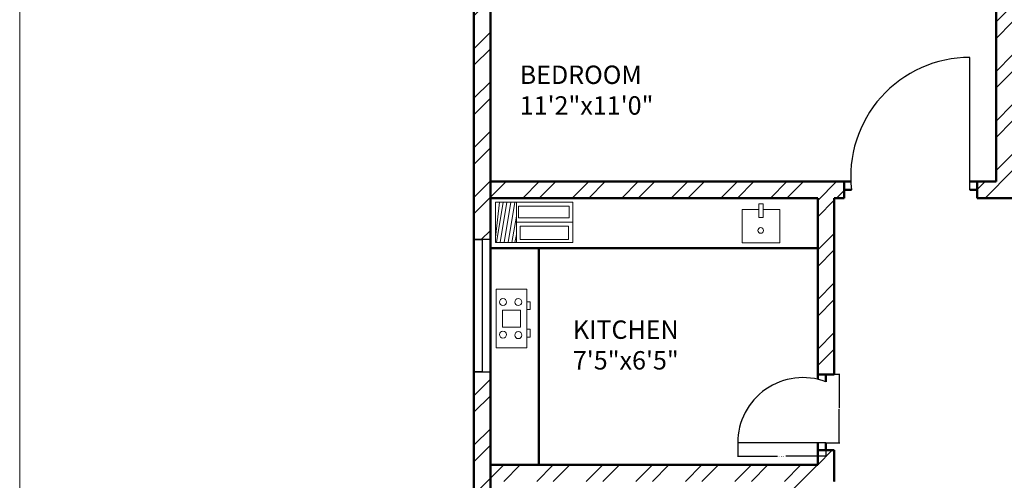
# Model space of a CAD drawing. Units: inches. Extents: x 1901 to 2863, y 888 to 2433.
# Tile 54 of 91: x 1901 to 2169, y 2002 to 2127. Entities that reach past the tile are written whole.
import ezdxf

# ---------------------------------------------------------------- set-up
doc = ezdxf.new("R2010")
doc.units = ezdxf.units.IN
for name, color, linetype, lineweight in [('A-ANNO-DIMS', 2, 'Continuous', 18), ('A-AREA-IDEN', 7, 'Continuous', 18), ('A-DOOR', 4, 'Continuous', 25), ('A-FLOR-FIXT', 9, 'Continuous', 18), ('A-GLAZ', 3, 'Continuous', 25), ('A-WALL', 7, 'Continuous', 50), ('A-WALL-PATT', 8, 'Continuous', 13)]:
    doc.layers.add(name, color=color, linetype=linetype, lineweight=lineweight)
doc.styles.get("Standard").update_dxf_attribs({"font": 'arial.ttf'})
doc.dimstyles.get("Standard").update_dxf_attribs({"dimtxt": 0.18, "dimasz": 0.18, "dimexe": 0.18, "dimexo": 0.0625, "dimgap": 0.09, "dimtad": 0, "dimtih": 1, "dimtoh": 1, "dimdec": 4, "dimzin": 0, "dimdsep": 46, "dimtxsty": 'Standard', "dimcen": 0.09, "dimadec": 0, "dimazin": 0, "dimtfac": 1, "dimtdec": 4, "dimtofl": 0, "dimtmove": 0, "dimatfit": 3, "dimfxl": 1, "dimtolj": 1, "dimtzin": 0, "dimarcsym": 0})

# ---------------------------------------------------------------- blocks, each defined once
blk = doc.blocks.new('WIN-36')
for p, q in [((4.5, 36), (0, 36)), ((0, 36), (2.25, 36)), ((2.25, 36), (2.25, 0)), ((2.25, 0), (0, 0)), ((0, 0), (4.5, 0))]:
    blk.add_line(p, q)
blk = doc.blocks.new('DOOR-18')
blk.add_line((23.98, -0.01), (-0.02, -0.01))
blk.add_arc((17.74, -0.01), 17.76, 69.4255, 180)
blk = doc.blocks.new('*D41')
at = {"layer": 'A-ANNO-DIMS', "color": 0, "lineweight": -2, "transparency": 16777216}
for p, q in [((2096.68, 2012.03), (2096.68, 2008.31)), ((2120.68, 2012.03), (2120.68, 2008.31)), ((2096.86, 2008.49), (2107.54, 2008.49)), ((2120.5, 2008.49), (2109.81, 2008.49))]:
    blk.add_line(p, q, dxfattribs=at)
at = {"layer": 'A-ANNO-DIMS', "color": 0, "transparency": 16777216}
for points in [[(2096.86, 2008.52), (2096.86, 2008.46), (2096.68, 2008.49)], [(2120.5, 2008.52), (2120.5, 2008.46), (2120.68, 2008.49)]]:
    blk.add_solid(points, dxfattribs=at)
at = {"layer": 'Defpoints', "color": 0, "transparency": 16777216}
for p in [(2096.68, 2012.09), (2120.68, 2012.09), (2120.68, 2008.49)]:
    blk.add_point(p, dxfattribs=at)
at = {"layer": 'A-ANNO-DIMS', "color": 0, "transparency": 16777216, "insert": (2108.68, 2008.49), "char_height": 0.18, "attachment_point": 5}
blk.add_mtext('\\A1;DOOR D6 24 TYP.', dxfattribs=at)
blk = doc.blocks.new('*D42')
at = {"layer": 'A-ANNO-DIMS', "color": 0, "lineweight": -2, "transparency": 16777216}
for p, q in [((2120.74, 2030.76), (2124.46, 2030.76)), ((2124.28, 2030.58), (2124.28, 2021.61)), ((2124.28, 2012.27), (2124.28, 2021.24)), ((2120.74, 2012.09), (2124.46, 2012.09))]:
    blk.add_line(p, q, dxfattribs=at)
at = {"layer": 'A-ANNO-DIMS', "color": 0, "transparency": 16777216}
for points in [[(2124.25, 2030.58), (2124.31, 2030.58), (2124.28, 2030.76)], [(2124.25, 2012.27), (2124.31, 2012.27), (2124.28, 2012.09)]]:
    blk.add_solid(points, dxfattribs=at)
at = {"layer": 'Defpoints', "color": 0, "transparency": 16777216}
for p in [(2120.68, 2030.76), (2124.28, 2030.76), (2120.68, 2012.09)]:
    blk.add_point(p, dxfattribs=at)
at = {"layer": 'A-ANNO-DIMS', "color": 0, "transparency": 16777216, "insert": (2124.28, 2021.43), "char_height": 0.18, "attachment_point": 5}
blk.add_mtext('\\A1;19 TYP.', dxfattribs=at)

msp = doc.modelspace()

# ---------------------------------------------------------------- hatches: boundary and pattern name
at = {"layer": 'A-WALL-PATT'}
h = msp.add_hatch(dxfattribs=at)
h.set_pattern_fill('ANSI32', color=256)
h.paths.add_polyline_path([(2192.5, 2274.13), (2141.26, 2274.13), (2141.26, 2269.63), (2192.5, 2269.63)])
h.paths.add_polyline_path([(2259.93, 2274.13), (2216.5, 2274.13), (2216.5, 2269.63), (2255.43, 2269.63), (2255.43, 2214.63), (2250.81, 2214.63), (2250.81, 2210.13), (2259.93, 2210.13), (2259.93, 2215.13), (2271.76, 2215.13), (2271.76, 2217.38), (2271.76, 2219.63), (2259.93, 2219.63)])
h.paths.add_polyline_path([(2171.43, 2269.63), (2166.93, 2269.63), (2166.93, 2219.63), (2121.24, 2219.63), (2121.24, 2215.13), (2166.93, 2215.13), (2166.93, 2083.13), (2161.81, 2083.13), (2161.81, 2078.63), (2171.43, 2078.63), (2177, 2078.63), (2177, 2080.88), (2177, 2083.13), (2171.43, 2083.13), (2171.43, 2210.13), (2230.91, 2210.13), (2230.91, 2212.38), (2230.91, 2214.63), (2171.43, 2214.63)])
h.paths.add_polyline_path([(2117.26, 2274.13), (2089.43, 2274.13), (2089.43, 2219.63), (2081.14, 2219.63), (2081.14, 2215.13), (2089.43, 2215.13), (2098, 2215.13), (2098, 2217.38), (2098, 2219.63), (2093.93, 2219.63), (2093.93, 2269.63), (2117.26, 2269.63), (2117.26, 2271.88)])
h.paths.add_polyline_path([(2343.43, 2219.63), (2329.29, 2219.63), (2329.29, 2215.13), (2338.93, 2215.13), (2338.93, 2184.74), (2343.43, 2184.74)])
h.paths.add_polyline_path([(2338.93, 2083.13), (2329.29, 2083.13), (2208.97, 2083.13), (2208.97, 2078.63), (2338.93, 2078.63)])
h.paths.add_polyline_path([(2343.43, 2136.74), (2338.93, 2136.74), (2338.93, 1872.63), (2343.43, 1872.63)])
h.paths.add_polyline_path([(2343.43, 1863.63), (2397.68, 1863.63), (2397.68, 1821.63), (2384.14, 1821.63), (2384.14, 1812.63), (2418.33, 1812.63), (2418.33, 1817.13), (2418.33, 1821.63), (2406.68, 1821.63), (2406.68, 1863.63), (2459.5, 1863.63), (2459.5, 1821.63), (2447.14, 1821.63), (2447.14, 1812.63), (2459.5, 1812.63), (2468.5, 1812.63), (2468.5, 1872.63), (2394.43, 1872.63), (2334.43, 1872.63), (2334.43, 1812.63), (2343.43, 1812.63), (2353.25, 1812.63), (2353.25, 1821.63), (2343.43, 1821.63)])
h.paths.add_polyline_path([(2510.01, 1872.63), (2468.5, 1872.63), (2468.5, 1868.13), (2510.01, 1868.13)])
h.paths.add_polyline_path([(2514.01, 1817.13), (2468.5, 1817.13), (2468.5, 1812.63), (2482.11, 1812.63), (2482.11, 1800.61), (2486.61, 1800.61), (2486.61, 1812.63), (2514.01, 1812.63)])
h.paths.add_polyline_path([(2299.25, 1814.88), (2299.25, 1817.13), (2295.93, 1817.13), (2295.93, 1854.17), (2293.68, 1854.17), (2291.43, 1854.17), (2291.43, 1817.13), (2266.11, 1817.13), (2266.11, 1812.63), (2299.25, 1812.63)])
h.paths.add_polyline_path([(2218.11, 1817.13), (2206.46, 1817.13), (2171.43, 1817.13), (2171.43, 1949.13), (2190.1, 1949.13), (2190.1, 1953.63), (2163.47, 1953.63), (2163.47, 1949.13), (2166.93, 1949.13), (2166.93, 1817.13), (2114.3, 1817.13), (2114.3, 1812.63), (2218.11, 1812.63)])
h.paths.add_polyline_path([(2029.43, 1970.92), (2024.93, 1970.92), (2024.93, 1912.72), (2029.43, 1912.72)])
h.paths.add_polyline_path([(2132.3, 1953.63), (2113.93, 1953.63), (2113.93, 1975.89), (2111.68, 1975.89), (2109.43, 1975.89), (2109.43, 1953.63), (2029.43, 1953.63), (2029.43, 1949.13), (2132.3, 1949.13)])
h.paths.add_polyline_path([(2029.43, 1853.61), (2029.31, 1853.61), (2029.31, 1853.61), (2029.43, 1853.61), (2029.43, 1864.72), (2024.93, 1864.72), (2024.93, 1812.63), (2066.3, 1812.63), (2066.3, 1814.88), (2066.3, 1817.13), (2029.43, 1817.13)])
h.paths.add_polyline_path([(2122.93, 2010.09), (2120.68, 2010.09), (2118.43, 2010.09), (2118.43, 2006.13), (2029.43, 2006.13), (2029.43, 2001.63), (2109.43, 2001.63), (2109.43, 1998.04), (2113.93, 1998.04), (2113.93, 2001.63), (2122.93, 2001.63)])
h.paths.add_polyline_path([(2029.43, 2031.38), (2024.93, 2031.38), (2024.93, 1994.92), (2027.18, 1994.92), (2029.43, 1994.92)])
h.paths.add_polyline_path([(2029.43, 2136.74), (2024.93, 2136.74), (2024.93, 2067.38), (2027.18, 2067.38), (2029.43, 2067.38)])
h.paths.add_polyline_path([(2125.62, 2083.13), (2029.43, 2083.13), (2029.43, 2078.63), (2118.43, 2078.63), (2118.43, 2030.71), (2122.93, 2030.71), (2122.93, 2078.63), (2125.62, 2078.63)])
h.paths.add_polyline_path([(2029.43, 2215.13), (2040.47, 2215.13), (2040.47, 2217.38), (2040.47, 2219.63), (2024.93, 2219.63), (2024.93, 2184.74), (2029.43, 2184.74), (2029.43, 2187.78)])
h.paths.add_polyline_path([(2686.43, 2274.13), (2659.28, 2274.13), (2659.28, 2269.63), (2681.93, 2269.63), (2681.93, 2219.63), (2676.82, 2219.63), (2676.82, 2215.13), (2681.93, 2215.13), (2697.01, 2215.13), (2697.01, 2217.38), (2697.01, 2219.63), (2686.43, 2219.63)])
h.paths.add_polyline_path([(2609.93, 2269.63), (2635.28, 2269.63), (2635.28, 2274.13), (2571.43, 2274.13), (2571.43, 2269.63), (2605.43, 2269.63), (2605.43, 2214.63), (2549.1, 2214.63), (2549.1, 2210.13), (2605.43, 2210.13), (2605.43, 2083.13), (2601.01, 2083.13), (2601.01, 2080.88), (2601.01, 2078.63), (2609.93, 2078.63), (2616.16, 2078.63), (2616.16, 2080.88), (2616.16, 2083.13), (2609.93, 2083.13), (2609.93, 2215.13), (2651.46, 2215.13), (2651.46, 2217.38), (2651.46, 2219.63), (2609.93, 2219.63)])
h.paths.add_polyline_path([(2521.43, 2269.63), (2547.43, 2269.63), (2547.43, 2271.88), (2547.43, 2274.13), (2516.93, 2274.13), (2516.93, 2219.63), (2506.41, 2219.63), (2506.41, 2215.13), (2516.93, 2215.13), (2516.93, 2210.13), (2525.4, 2210.13), (2525.4, 2212.38), (2525.4, 2214.63), (2521.43, 2214.63)])
h.paths.add_polyline_path([(2456.01, 2219.63), (2439.43, 2219.63), (2439.43, 2187.89), (2443.93, 2187.89), (2443.93, 2215.13), (2456.01, 2215.13)])
h.paths.add_polyline_path([(2752.93, 2219.63), (2739.48, 2219.63), (2739.48, 2215.13), (2748.43, 2215.13), (2748.43, 2187.89), (2752.93, 2187.89)])
h.paths.add_polyline_path([(2752.93, 2139.89), (2748.43, 2139.89), (2748.43, 2083.13), (2648.42, 2083.13), (2648.42, 2078.63), (2654.93, 2078.63), (2654.93, 2039.44), (2659.43, 2039.44), (2659.43, 2078.63), (2748.43, 2078.63), (2748.43, 2063.43), (2752.93, 2063.43)])
h.paths.add_polyline_path([(2752.93, 2010.63), (2659.43, 2010.63), (2659.43, 2015.65), (2654.93, 2015.65), (2654.93, 2010.63), (2605.43, 2010.63), (2605.43, 1920.97), (2609.93, 1920.97), (2609.93, 2006.13), (2748.43, 2006.13), (2748.43, 1982.47), (2752.93, 1982.47)])
h.paths.add_polyline_path([(2752.93, 2027.43), (2748.43, 2027.43), (2748.43, 2010.63), (2752.93, 2010.63)])
h.paths.add_polyline_path([(2748.43, 1886.13), (2609.93, 1886.13), (2609.93, 1889.72), (2605.43, 1889.72), (2605.43, 1861.26), (2609.93, 1861.26), (2609.93, 1881.63), (2748.43, 1881.63)])
h.paths.add_polyline_path([(2456.86, 2228.83), (2498.4, 2228.83), (2498.4, 2247.49), (2456.86, 2247.49)], flags=9)
h.paths.add_polyline_path([(2038.6, 2237.42), (2080.17, 2237.42), (2080.17, 2256.08), (2038.6, 2256.08)], flags=9)
h.paths.add_polyline_path([(2292.01, 1062.39), (2539.93, 1062.39), (2539.93, 1099.49), (2292.01, 1099.49)], flags=9)
h.paths.add_polyline_path([(2424.91, 1832.25), (2448.51, 1832.25), (2448.51, 1846.68), (2424.91, 1846.68)], flags=25)
h.paths.add_polyline_path([(2359.08, 1832.25), (2382.68, 1832.25), (2382.68, 1846.68), (2359.08, 1846.68)], flags=25)
h.paths.add_polyline_path([(2352.9, 1684.8), (2367.54, 1684.8), (2367.54, 1697.17), (2352.9, 1697.17)], flags=9)
h.paths.add_polyline_path([(2079.29, 1755.83), (2169.02, 1755.83), (2169.02, 1774.37), (2079.29, 1774.37)], flags=9)
h.paths.add_polyline_path([(2404.09, 1373.86), (2404.09, 1463.59), (2385.54, 1463.59), (2385.54, 1373.86)], flags=9)
h.paths.add_polyline_path([(2268.09, 2236.37), (2309.64, 2236.37), (2309.64, 2255.03), (2268.09, 2255.03)], flags=9)
h.paths.add_polyline_path([(2575.96, 1700.95), (2665.7, 1700.95), (2665.7, 1719.5), (2575.96, 1719.5)], flags=9)
h.paths.add_polyline_path([(2302.96, 1878.47), (2329.52, 1878.47), (2329.52, 1888.78), (2302.96, 1888.78)], flags=9)
h.paths.add_polyline_path([(2097.42, 2240.58), (2126.57, 2240.58), (2126.57, 2259.23), (2097.42, 2259.23)], flags=9)
h.paths.add_polyline_path([(2208.72, 2246.12), (2237.88, 2246.12), (2237.88, 2264.78), (2208.72, 2264.78)], flags=9)
h.paths.add_polyline_path([(2038.15, 1925.96), (2076.99, 1925.96), (2076.99, 1944.62), (2038.15, 1944.62)], flags=9)
h.paths.add_polyline_path([(2239.14, 1926.67), (2288.46, 1926.67), (2288.46, 1945.33), (2239.14, 1945.33)], flags=9)
h.paths.add_polyline_path([(2175.43, 2007.33), (2212.36, 2007.33), (2212.36, 2025.99), (2175.43, 2025.99)], flags=9)
h.paths.add_polyline_path([(2225.03, 2091.79), (2263.87, 2091.79), (2263.87, 2110.45), (2225.03, 2110.45)], flags=9)
h.paths.add_polyline_path([(2035.4, 2098.48), (2074.24, 2098.48), (2074.24, 2117.14), (2035.4, 2117.14)], flags=9)
h.paths.add_polyline_path([(2050.1, 2029.21), (2083.26, 2029.21), (2083.26, 2047.87), (2050.1, 2047.87)], flags=9)
h.paths.add_polyline_path([(2069.68, 1956.72), (2098.83, 1956.72), (2098.83, 1975.38), (2069.68, 1975.38)], flags=25)
h.paths.add_polyline_path([(2328.62, 1753.34), (2361.66, 1753.34), (2361.66, 1771.99), (2328.62, 1771.99)], flags=9)
h.paths.add_polyline_path([(2395.16, 2060.89), (2395.16, 2140.65), (2378.68, 2140.65), (2378.68, 2060.89)], flags=9)
h.paths.add_polyline_path([(2463.73, 2059.02), (2492.89, 2059.02), (2492.89, 2077.68), (2463.73, 2077.68)], flags=9)
h.paths.add_polyline_path([(2458.03, 2181.54), (2496.87, 2181.54), (2496.87, 2200.19), (2458.03, 2200.19)], flags=9)
h.paths.add_polyline_path([(2527.58, 2243.07), (2556.73, 2243.07), (2556.73, 2261.73), (2527.58, 2261.73)], flags=9)
h.paths.add_polyline_path([(2694.46, 2232.77), (2736.03, 2232.77), (2736.03, 2251.42), (2694.46, 2251.42)], flags=9)
h.paths.add_polyline_path([(2637.82, 2249.22), (2666.98, 2249.22), (2666.98, 2267.88), (2637.82, 2267.88)], flags=9)
h.paths.add_polyline_path([(2623.69, 2183.54), (2662.53, 2183.54), (2662.53, 2202.2), (2623.69, 2202.2)], flags=9)
h.paths.add_polyline_path([(2691.97, 2021.5), (2725.12, 2021.5), (2725.12, 2040.16), (2691.97, 2040.16)], flags=9)
h.paths.add_polyline_path([(2621.04, 1975.91), (2662.34, 1975.91), (2662.34, 1994.57), (2621.04, 1994.57)], flags=25)
h.paths.add_polyline_path([(2479.03, 1927.62), (2519.84, 1927.62), (2519.84, 1946.28), (2479.03, 1946.28)], flags=9)
h.paths.add_polyline_path([(2670.94, 1849.08), (2716.01, 1849.08), (2716.01, 1867.73), (2670.94, 1867.73)], flags=9)
h.paths.add_polyline_path([(2523.61, 1782.96), (2550.17, 1782.96), (2550.17, 1793.26), (2523.61, 1793.26)], flags=9)
h.paths.add_polyline_path([(2450.84, 1207.33), (2492.39, 1207.33), (2492.39, 1225.99), (2450.84, 1225.99)], flags=9)
h.paths.add_polyline_path([(2527.75, 1203.84), (2556.91, 1203.84), (2556.91, 1222.5), (2527.75, 1222.5)], flags=9)
h.paths.add_polyline_path([(2639.11, 1207.2), (2668.27, 1207.2), (2668.27, 1225.86), (2639.11, 1225.86)], flags=9)
h.paths.add_polyline_path([(2692.59, 1218.97), (2734.17, 1218.97), (2734.17, 1237.62), (2692.59, 1237.62)], flags=9)
h.paths.add_polyline_path([(2669.27, 1366.33), (2708.11, 1366.33), (2708.11, 1384.99), (2669.27, 1384.99)], flags=9)
h.paths.add_polyline_path([(2463.31, 1358.03), (2502.15, 1358.03), (2502.15, 1376.69), (2463.31, 1376.69)], flags=9)
h.paths.add_polyline_path([(2494.72, 1449.96), (2531.65, 1449.96), (2531.65, 1468.62), (2494.72, 1468.62)], flags=9)
h.paths.add_polyline_path([(2675.57, 1422.16), (2708.72, 1422.16), (2708.72, 1440.81), (2675.57, 1440.81)], flags=9)
h.paths.add_polyline_path([(2685.63, 1493.89), (2714.79, 1493.89), (2714.79, 1512.55), (2685.63, 1512.55)], flags=9)
h.paths.add_polyline_path([(2686.8, 1529.91), (2725.65, 1529.91), (2725.65, 1548.57), (2686.8, 1548.57)], flags=9)
h.paths.add_polyline_path([(2503.65, 1537.99), (2552.97, 1537.99), (2552.97, 1556.65), (2503.65, 1556.65)], flags=9)
h.paths.add_polyline_path([(2291.71, 1643.5), (2318.28, 1643.5), (2318.28, 1653.81), (2291.71, 1653.81)], flags=9)
h.paths.add_polyline_path([(2450.63, 1610.52), (2477.19, 1610.52), (2477.19, 1620.82), (2450.63, 1620.82)], flags=9)
h.paths.add_polyline_path([(2359.99, 1551.81), (2422.25, 1551.81), (2422.25, 1562.12), (2359.99, 1562.12)], flags=9)
h.paths.add_polyline_path([(2280.11, 1249.01), (2321.65, 1249.01), (2321.65, 1267.66), (2280.11, 1267.66)], flags=9)
h.paths.add_polyline_path([(2164.06, 1274.23), (2193.22, 1274.23), (2193.22, 1292.89), (2164.06, 1292.89)], flags=9)
h.paths.add_polyline_path([(2118.21, 1277.69), (2151.25, 1277.69), (2151.25, 1296.35), (2118.21, 1296.35)], flags=9)
h.paths.add_polyline_path([(2031.95, 1268.53), (2073.52, 1268.53), (2073.52, 1287.19), (2031.95, 1287.19)], flags=9)
h.paths.add_polyline_path([(2050.2, 1409.08), (2089.04, 1409.08), (2089.04, 1427.74), (2050.2, 1427.74)], flags=9)
h.paths.add_polyline_path([(2243.74, 1421.03), (2282.58, 1421.03), (2282.58, 1439.69), (2243.74, 1439.69)], flags=9)
h.paths.add_polyline_path([(2190.75, 1509.77), (2231.56, 1509.77), (2231.56, 1528.43), (2190.75, 1528.43)], flags=9)
h.paths.add_polyline_path([(2058.39, 1475.42), (2091.55, 1475.42), (2091.55, 1494.07), (2058.39, 1494.07)], flags=9)
h.paths.add_polyline_path([(2062.45, 1553.09), (2091.6, 1553.09), (2091.6, 1571.75), (2062.45, 1571.75)], flags=9)
h.paths.add_polyline_path([(2219.52, 1590.37), (2266.15, 1590.37), (2266.15, 1609.02), (2219.52, 1609.02)], flags=9)
h.paths.add_polyline_path([(2041.07, 1584.19), (2079.91, 1584.19), (2079.91, 1602.85), (2041.07, 1602.85)], flags=9)
h = msp.add_hatch(dxfattribs=at)
h.set_pattern_fill('ANSI32', color=256)
h.paths.add_polyline_path([(2443.93, 2139.89), (2439.43, 2139.89), (2439.43, 2069.35), (2441.68, 2069.35), (2443.93, 2069.35), (2443.93, 2078.63), (2521.93, 2078.63), (2521.93, 2075.07), (2524.18, 2075.07), (2526.43, 2075.07), (2526.43, 2078.63), (2571.75, 2078.63), (2571.75, 2080.88), (2571.75, 2083.13), (2443.93, 2083.13)])
h.paths.add_polyline_path([(2526.43, 2054.63), (2524.18, 2054.63), (2521.93, 2054.63), (2521.93, 2030.63), (2443.93, 2030.63), (2443.93, 2045.35), (2439.43, 2045.35), (2439.43, 1983.87), (2443.93, 1983.87), (2443.93, 2026.13), (2521.93, 2026.13), (2526.43, 2026.13)])
h.paths.add_polyline_path([(2443.93, 1923.87), (2439.43, 1923.87), (2439.43, 1872.63), (2443.93, 1872.63)])
h.paths.add_polyline_path([(2636.23, 1766.13), (2609.93, 1766.13), (2609.93, 1779.79), (2605.43, 1779.79), (2605.43, 1766.13), (2486.61, 1766.13), (2486.61, 1770.67), (2482.11, 1770.67), (2482.11, 1766.13), (2482.11, 1761.63), (2636.23, 1761.63), (2636.23, 1763.88)])
h.paths.add_polyline_path([(2519.54, 1663.38), (2519.54, 1665.63), (2494.93, 1665.63), (2481.83, 1665.63), (2481.83, 1663.38), (2481.83, 1661.13), (2490.43, 1661.13), (2490.43, 1640.16), (2494.93, 1640.16), (2494.93, 1661.13), (2519.54, 1661.13)])
h.paths.add_polyline_path([(2443.93, 1712.13), (2443.93, 1716.63), (2414.46, 1716.63), (2414.46, 1712.13), (2439.43, 1712.13), (2439.43, 1545.51), (2443.93, 1545.51), (2443.93, 1661.13), (2448.47, 1661.13), (2448.47, 1665.63), (2443.93, 1665.63)])
h.paths.add_polyline_path([(2343.43, 1712.13), (2365.52, 1712.13), (2365.52, 1714.38), (2365.52, 1716.63), (2333.87, 1716.63), (2333.87, 1714.38), (2333.87, 1712.13), (2338.93, 1712.13), (2338.93, 1575.63), (2338.93, 1545.51), (2343.43, 1545.51), (2343.43, 1547.51), (2343.43, 1580.13)])
h.paths.add_polyline_path([(2752.93, 1665.63), (2579.54, 1665.63), (2579.54, 1661.13), (2615.93, 1661.13), (2615.93, 1529.13), (2598.93, 1529.13), (2598.93, 1524.63), (2623.13, 1524.63), (2623.13, 1526.88), (2623.13, 1529.13), (2620.43, 1529.13), (2620.43, 1661.13), (2748.43, 1661.13), (2748.43, 1633.5), (2752.93, 1633.5)])
h.paths.add_polyline_path([(2752.93, 1419.93), (2748.43, 1419.93), (2748.43, 1400.13), (2659.43, 1400.13), (2659.43, 1444.33), (2657.18, 1444.33), (2654.93, 1444.33), (2654.93, 1400.13), (2643.65, 1400.13), (2643.65, 1395.63), (2748.43, 1395.63), (2748.43, 1364.04), (2752.93, 1364.04)])
h.paths.add_polyline_path([(2752.93, 1492.88), (2748.43, 1492.88), (2748.43, 1476.63), (2667.43, 1476.63), (2667.43, 1479.71), (2665.18, 1479.71), (2662.93, 1479.71), (2662.93, 1476.63), (2654.93, 1476.63), (2654.93, 1469.54), (2659.43, 1469.54), (2659.43, 1472.13), (2748.43, 1472.13), (2748.43, 1455.93), (2752.93, 1455.93)])
h.paths.add_polyline_path([(2752.93, 1304.04), (2748.43, 1304.04), (2748.43, 1263.63), (2738.66, 1263.63), (2738.66, 1259.13), (2752.93, 1259.13)])
h.paths.add_polyline_path([(2685.93, 1259.13), (2695.49, 1259.13), (2695.49, 1261.38), (2695.49, 1263.63), (2677.84, 1263.63), (2677.84, 1261.38), (2677.84, 1259.13), (2681.43, 1259.13), (2681.43, 1203.63), (2653.28, 1203.63), (2653.28, 1199.13), (2685.93, 1199.13), (2685.93, 1203.63)])
h.paths.add_polyline_path([(2609.43, 1395.63), (2611.85, 1395.63), (2611.85, 1400.13), (2598.89, 1400.13), (2598.89, 1397.88), (2598.89, 1395.63), (2604.93, 1395.63), (2604.93, 1268.13), (2554.73, 1268.13), (2554.73, 1265.88), (2554.73, 1263.63), (2604.93, 1263.63), (2604.93, 1203.63), (2571.31, 1203.63), (2571.31, 1199.13), (2604.93, 1199.13), (2629.28, 1199.13), (2629.28, 1201.38), (2629.28, 1203.63), (2609.43, 1203.63), (2609.43, 1258.63), (2609.43, 1259.13), (2654.8, 1259.13), (2654.8, 1263.63), (2609.43, 1263.63)])
h.paths.add_polyline_path([(2443.93, 1304.04), (2439.43, 1304.04), (2439.43, 1259.13), (2443.93, 1259.13), (2456.16, 1259.13), (2456.16, 1261.38), (2456.16, 1263.63), (2443.93, 1263.63)])
h.paths.add_polyline_path([(2525.43, 1263.63), (2531.78, 1263.63), (2531.78, 1268.13), (2520.93, 1268.13), (2520.93, 1263.63), (2511.41, 1263.63), (2511.41, 1259.13), (2520.93, 1259.13), (2520.93, 1199.13), (2547.31, 1199.13), (2547.31, 1201.38), (2547.31, 1203.63), (2525.43, 1203.63)])
h.paths.add_polyline_path([(2443.93, 1434.84), (2439.43, 1434.84), (2439.43, 1364.04), (2441.68, 1364.04), (2443.93, 1364.04)])
h.paths.add_polyline_path([(2567.13, 1400.13), (2443.93, 1400.13), (2443.93, 1395.63), (2567.13, 1395.63)])
h.paths.add_polyline_path([(2443.93, 1545.51), (2439.43, 1545.51), (2439.43, 1494.84), (2443.93, 1494.84)])
h.paths.add_polyline_path([(2494.93, 1553.35), (2492.68, 1553.35), (2490.43, 1553.35), (2490.43, 1524.63), (2494.93, 1524.63), (2525.94, 1524.63), (2525.94, 1526.88), (2525.94, 1529.13), (2494.93, 1529.13)])
h.paths.add_polyline_path([(2752.93, 1573.5), (2748.43, 1573.5), (2748.43, 1529.13), (2657.76, 1529.13), (2657.76, 1524.63), (2662.93, 1524.63), (2662.93, 1498.63), (2667.43, 1498.63), (2667.43, 1524.63), (2748.43, 1524.63), (2748.43, 1516.88), (2752.93, 1516.88)])
h.paths.add_polyline_path([(2038.6, 2237.42), (2080.17, 2237.42), (2080.17, 2256.08), (2038.6, 2256.08)], flags=9)
h.paths.add_polyline_path([(2292.01, 1062.39), (2539.93, 1062.39), (2539.93, 1099.49), (2292.01, 1099.49)], flags=9)
h.paths.add_polyline_path([(2424.91, 1832.25), (2448.51, 1832.25), (2448.51, 1846.68), (2424.91, 1846.68)], flags=9)
h.paths.add_polyline_path([(2359.08, 1832.25), (2382.68, 1832.25), (2382.68, 1846.68), (2359.08, 1846.68)], flags=9)
h.paths.add_polyline_path([(2352.9, 1684.8), (2367.54, 1684.8), (2367.54, 1697.17), (2352.9, 1697.17)], flags=9)
h.paths.add_polyline_path([(2079.29, 1755.83), (2169.02, 1755.83), (2169.02, 1774.37), (2079.29, 1774.37)], flags=9)
h.paths.add_polyline_path([(2404.09, 1373.86), (2404.09, 1463.59), (2385.54, 1463.59), (2385.54, 1373.86)], flags=9)
h.paths.add_polyline_path([(2268.09, 2236.37), (2309.64, 2236.37), (2309.64, 2255.03), (2268.09, 2255.03)], flags=9)
h.paths.add_polyline_path([(2575.96, 1700.95), (2665.7, 1700.95), (2665.7, 1719.5), (2575.96, 1719.5)], flags=9)
h.paths.add_polyline_path([(2302.96, 1878.47), (2329.52, 1878.47), (2329.52, 1888.78), (2302.96, 1888.78)], flags=9)
h.paths.add_polyline_path([(2097.42, 2240.58), (2126.57, 2240.58), (2126.57, 2259.23), (2097.42, 2259.23)], flags=9)
h.paths.add_polyline_path([(2208.72, 2246.12), (2237.88, 2246.12), (2237.88, 2264.78), (2208.72, 2264.78)], flags=9)
h.paths.add_polyline_path([(2038.15, 1925.96), (2076.99, 1925.96), (2076.99, 1944.62), (2038.15, 1944.62)], flags=9)
h.paths.add_polyline_path([(2239.14, 1926.67), (2288.46, 1926.67), (2288.46, 1945.33), (2239.14, 1945.33)], flags=9)
h.paths.add_polyline_path([(2175.43, 2007.33), (2212.36, 2007.33), (2212.36, 2025.99), (2175.43, 2025.99)], flags=9)
h.paths.add_polyline_path([(2225.03, 2091.79), (2263.87, 2091.79), (2263.87, 2110.45), (2225.03, 2110.45)], flags=9)
h.paths.add_polyline_path([(2035.4, 2098.48), (2074.24, 2098.48), (2074.24, 2117.14), (2035.4, 2117.14)], flags=9)
h.paths.add_polyline_path([(2050.1, 2029.21), (2083.26, 2029.21), (2083.26, 2047.87), (2050.1, 2047.87)], flags=9)
h.paths.add_polyline_path([(2069.68, 1956.72), (2098.83, 1956.72), (2098.83, 1975.38), (2069.68, 1975.38)], flags=9)
h.paths.add_polyline_path([(2328.62, 1753.34), (2361.66, 1753.34), (2361.66, 1771.99), (2328.62, 1771.99)], flags=9)
h.paths.add_polyline_path([(2395.16, 2060.89), (2395.16, 2140.65), (2378.68, 2140.65), (2378.68, 2060.89)], flags=9)
h.paths.add_polyline_path([(2463.73, 2059.02), (2492.89, 2059.02), (2492.89, 2077.68), (2463.73, 2077.68)], flags=9)
h.paths.add_polyline_path([(2458.03, 2181.54), (2496.87, 2181.54), (2496.87, 2200.19), (2458.03, 2200.19)], flags=9)
h.paths.add_polyline_path([(2456.86, 2228.83), (2498.4, 2228.83), (2498.4, 2247.49), (2456.86, 2247.49)], flags=9)
h.paths.add_polyline_path([(2527.58, 2243.07), (2556.73, 2243.07), (2556.73, 2261.73), (2527.58, 2261.73)], flags=9)
h.paths.add_polyline_path([(2694.46, 2232.77), (2736.03, 2232.77), (2736.03, 2251.42), (2694.46, 2251.42)], flags=9)
h.paths.add_polyline_path([(2637.82, 2249.22), (2666.98, 2249.22), (2666.98, 2267.88), (2637.82, 2267.88)], flags=9)
h.paths.add_polyline_path([(2623.69, 2183.54), (2662.53, 2183.54), (2662.53, 2202.2), (2623.69, 2202.2)], flags=9)
h.paths.add_polyline_path([(2691.97, 2021.5), (2725.12, 2021.5), (2725.12, 2040.16), (2691.97, 2040.16)], flags=9)
h.paths.add_polyline_path([(2621.04, 1975.91), (2662.34, 1975.91), (2662.34, 1994.57), (2621.04, 1994.57)], flags=9)
h.paths.add_polyline_path([(2479.03, 1927.62), (2519.84, 1927.62), (2519.84, 1946.28), (2479.03, 1946.28)], flags=9)
h.paths.add_polyline_path([(2670.94, 1849.08), (2716.01, 1849.08), (2716.01, 1867.73), (2670.94, 1867.73)], flags=9)
h.paths.add_polyline_path([(2523.61, 1782.96), (2550.17, 1782.96), (2550.17, 1793.26), (2523.61, 1793.26)], flags=9)
h.paths.add_polyline_path([(2450.84, 1207.33), (2492.39, 1207.33), (2492.39, 1225.99), (2450.84, 1225.99)], flags=9)
h.paths.add_polyline_path([(2527.75, 1203.84), (2556.91, 1203.84), (2556.91, 1222.5), (2527.75, 1222.5)], flags=9)
h.paths.add_polyline_path([(2639.11, 1207.2), (2668.27, 1207.2), (2668.27, 1225.86), (2639.11, 1225.86)], flags=9)
h.paths.add_polyline_path([(2692.59, 1218.97), (2734.17, 1218.97), (2734.17, 1237.62), (2692.59, 1237.62)], flags=9)
h.paths.add_polyline_path([(2669.27, 1366.33), (2708.11, 1366.33), (2708.11, 1384.99), (2669.27, 1384.99)], flags=25)
h.paths.add_polyline_path([(2463.31, 1358.03), (2502.15, 1358.03), (2502.15, 1376.69), (2463.31, 1376.69)], flags=9)
h.paths.add_polyline_path([(2494.72, 1449.96), (2531.65, 1449.96), (2531.65, 1468.62), (2494.72, 1468.62)], flags=9)
h.paths.add_polyline_path([(2675.57, 1422.16), (2708.72, 1422.16), (2708.72, 1440.81), (2675.57, 1440.81)], flags=25)
h.paths.add_polyline_path([(2685.63, 1493.89), (2714.79, 1493.89), (2714.79, 1512.55), (2685.63, 1512.55)], flags=9)
h.paths.add_polyline_path([(2686.8, 1529.91), (2725.65, 1529.91), (2725.65, 1548.57), (2686.8, 1548.57)], flags=25)
h.paths.add_polyline_path([(2503.65, 1537.99), (2552.97, 1537.99), (2552.97, 1556.65), (2503.65, 1556.65)], flags=9)
h.paths.add_polyline_path([(2291.71, 1643.5), (2318.28, 1643.5), (2318.28, 1653.81), (2291.71, 1653.81)], flags=9)
h.paths.add_polyline_path([(2450.63, 1610.52), (2477.19, 1610.52), (2477.19, 1620.82), (2450.63, 1620.82)], flags=9)
h.paths.add_polyline_path([(2359.99, 1551.81), (2422.25, 1551.81), (2422.25, 1562.12), (2359.99, 1562.12)], flags=9)
h.paths.add_polyline_path([(2280.11, 1249.01), (2321.65, 1249.01), (2321.65, 1267.66), (2280.11, 1267.66)], flags=9)
h.paths.add_polyline_path([(2164.06, 1274.23), (2193.22, 1274.23), (2193.22, 1292.89), (2164.06, 1292.89)], flags=9)
h.paths.add_polyline_path([(2118.21, 1277.69), (2151.25, 1277.69), (2151.25, 1296.35), (2118.21, 1296.35)], flags=9)
h.paths.add_polyline_path([(2031.95, 1268.53), (2073.52, 1268.53), (2073.52, 1287.19), (2031.95, 1287.19)], flags=9)
h.paths.add_polyline_path([(2050.2, 1409.08), (2089.04, 1409.08), (2089.04, 1427.74), (2050.2, 1427.74)], flags=9)
h.paths.add_polyline_path([(2243.74, 1421.03), (2282.58, 1421.03), (2282.58, 1439.69), (2243.74, 1439.69)], flags=9)
h.paths.add_polyline_path([(2190.75, 1509.77), (2231.56, 1509.77), (2231.56, 1528.43), (2190.75, 1528.43)], flags=9)
h.paths.add_polyline_path([(2058.39, 1475.42), (2091.55, 1475.42), (2091.55, 1494.07), (2058.39, 1494.07)], flags=9)
h.paths.add_polyline_path([(2062.45, 1553.09), (2091.6, 1553.09), (2091.6, 1571.75), (2062.45, 1571.75)], flags=9)
h.paths.add_polyline_path([(2219.52, 1590.37), (2266.15, 1590.37), (2266.15, 1609.02), (2219.52, 1609.02)], flags=9)
h.paths.add_polyline_path([(2041.07, 1584.19), (2079.91, 1584.19), (2079.91, 1602.85), (2041.07, 1602.85)], flags=9)

# ---------------------------------------------------------------- linework, layer by layer
at = {"layer": 'A-DOOR'}
msp.add_line((2159.81, 2080.88), (2159.81, 2116.88), dxfattribs=at)
msp.add_arc((2159.81, 2084.49), 32.39, 90, 186.399, dxfattribs=at)
at = {"layer": 'A-FLOR-FIXT'}
for p, q in [((2031.92, 2077.55), (2030.79, 2067.96)), ((2032.93, 2077.55), (2031.1, 2066.57)), ((2033.93, 2077.55), (2031.92, 2077.55)), ((2033.93, 2077.55), (2032.06, 2066.57)), ((2035.03, 2077.55), (2033.19, 2066.57)), ((2036.09, 2077.55), (2034.25, 2066.57)), ((2036.51, 2077.55), (2036.51, 2066.57)), ((2036.51, 2077.55), (2036.51, 2077.55)), ((2036.51, 2073.74), (2035.29, 2066.57)), ((2036.51, 2072.06), (2051.9, 2072.06)), ((2036.51, 2068.71), (2036.05, 2066.57)), ((2035.74, 2066.57), (2033.93, 2066.57))]:
    msp.add_line(p, q, dxfattribs=at)
for points in [[(1901.45, 2433.12), (2863.43, 2433.12), (2863.43, 961.82), (1901.45, 961.82)], [(2030.79, 2077.55), (2051.9, 2077.55), (2051.9, 2066.57), (2030.79, 2066.57)], [(2037.08, 2076.46), (2050.84, 2076.46), (2050.84, 2073.24), (2037.08, 2073.24)], [(2102.44, 2077.05), (2103.57, 2077.05), (2103.57, 2073.36), (2102.44, 2073.36)], [(2037.56, 2071), (2050.64, 2071), (2050.64, 2067.39), (2037.56, 2067.39)], [(2030.99, 2053.85), (2039.34, 2053.85), (2039.34, 2037.93), (2030.99, 2037.93)], [(2032.71, 2048.19), (2037.58, 2048.19), (2037.58, 2043.53), (2032.71, 2043.53)], [(2039.34, 2050.47), (2040.29, 2050.47), (2040.29, 2048.35), (2039.34, 2048.35)], [(2039.34, 2043), (2040.29, 2043), (2040.29, 2040.88), (2039.34, 2040.88)]]:
    msp.add_lwpolyline(points, close=True, dxfattribs=at)
msp.add_lwpolyline([(2103.57, 2075.52), (2108.16, 2075.52), (2108.16, 2066.47), (2097.89, 2066.47), (2097.89, 2075.52), (2102.44, 2075.52)], dxfattribs=at)
for centre, radius in [((2102.93, 2069.84), 0.768), ((2032.86, 2050.38), 0.958), ((2037.02, 2050.38), 0.958), ((2032.86, 2041.54), 0.958), ((2037.03, 2041.39), 0.958)]:
    msp.add_circle(centre, radius, dxfattribs=at)
at = {"layer": 'A-WALL'}
for p, q in [((2024.93, 2219.63), (2024.93, 1812.63)), ((2029.43, 2215.13), (2029.43, 1817.13)), ((2166.93, 2215.13), (2166.93, 2083.13)), ((2029.43, 2083.13), (2127.45, 2083.13)), ((2081.14, 2083.13), (2089.43, 2083.13)), ((2125.62, 2078.63), (2125.62, 2083.13)), ((2125.62, 2083.13), (2125.62, 2080.88)), ((2159.81, 2083.13), (2166.93, 2083.13)), ((2161.81, 2083.13), (2161.81, 2078.63)), ((2125.62, 2080.88), (2127.62, 2080.88)), ((2161.81, 2080.88), (2159.81, 2080.88)), ((2161.81, 2078.63), (2161.81, 2080.88)), ((2029.43, 2078.63), (2118.43, 2078.63)), ((2029.43, 2078.63), (2118.43, 2078.63)), ((2118.43, 2078.63), (2118.43, 2029.39)), ((2122.93, 2030.71), (2122.93, 2078.63)), ((2122.93, 2078.63), (2125.62, 2078.63)), ((2161.81, 2078.63), (2171.43, 2078.63)), ((2042.64, 2064.99), (2029.43, 2064.99)), ((2042.64, 2006.13), (2042.64, 2064.99)), ((2042.64, 2064.99), (2118.43, 2064.99)), ((2118.43, 2030.71), (2122.93, 2030.71)), ((2122.93, 2030.71), (2120.68, 2030.71)), ((2120.68, 2030.71), (2120.68, 2028.71)), ((2118.43, 2012.09), (2118.43, 2006.13)), ((2120.68, 2010.09), (2120.68, 2012.09)), ((2118.43, 2010.09), (2122.93, 2010.09)), ((2122.93, 2010.09), (2120.68, 2010.09)), ((2122.93, 2001.63), (2122.93, 2010.09)), ((2029.43, 2006.13), (2118.43, 2006.13))]:
    msp.add_line(p, q, dxfattribs=at)

# ---------------------------------------------------------------- block references
at = {"layer": 'A-DOOR'}
msp.add_blockref('DOOR-18', (2096.7, 2012.1), dxfattribs=at)
at = {"layer": 'A-GLAZ'}
msp.add_blockref('WIN-36', (2024.93, 2031.38), dxfattribs=at)

# ---------------------------------------------------------------- texts
at = {"layer": 'A-AREA-IDEN', "char_height": 5, "attachment_point": 1}
for s, width, insert in [('BEDROOM\\P11\'2"x11\'0"', 232.77, (2037.41, 2114.65)), ('KITCHEN\\P7\'5"x6\'5"', 181.7671, (2051.86, 2045.38))]:
    msp.add_mtext_dynamic_manual_height_columns(s, width=width, gutter_width=12.5, heights=[0], dxfattribs=dict(at, insert=insert))

# ---------------------------------------------------------------- dimensions: what is measured, and where the dimension line sits
at = {"layer": 'A-ANNO-DIMS'}
dim = msp.add_linear_dim(base=(2124.28, 2030.76), p1=(2120.68, 2012.09), p2=(2120.68, 2030.76), angle=90, text='<> TYP.', dimstyle='Standard', override={"dimdec": 0, "dimlfac": 1, "dimrnd": 0, "dimzin": 0, "dimdsep": 46, "dimlunit": 2}, dxfattribs=at)
dim.commit()
dim.dimension.update_dxf_attribs({"geometry": '*D42', "text_midpoint": (2124.28, 2021.43)})
dim = msp.add_linear_dim(base=(2120.68, 2008.49), p1=(2096.68, 2012.09), p2=(2120.68, 2012.09), text='DOOR D6 <> TYP.', dimstyle='Standard', override={"dimdec": 0, "dimlfac": 1, "dimrnd": 0, "dimzin": 0, "dimdsep": 46, "dimlunit": 2}, dxfattribs=at)
dim.commit()
dim.dimension.update_dxf_attribs({"geometry": '*D41', "text_midpoint": (2108.68, 2008.49)})

doc.saveas('drawing.dxf')
